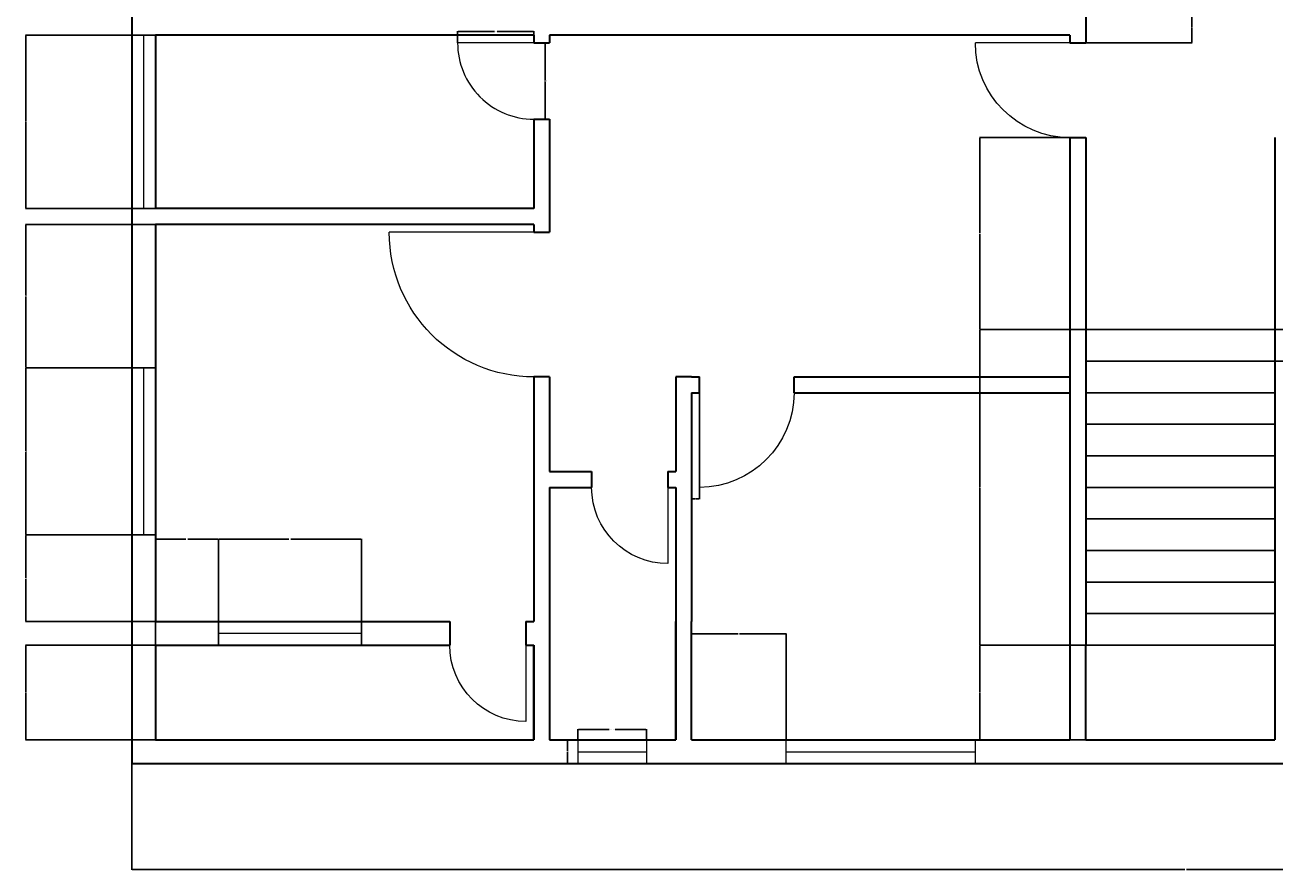
# Model space of a CAD drawing. Units: inches. Extents: x 2811 to 3694, y 2039 to 2670.
# Tile 1 of 3: x 2811 to 3286, y 2039 to 2361. Entities that reach past the tile are written whole.
import ezdxf

# ---------------------------------------------------------------- set-up
doc = ezdxf.new("R2010")
doc.units = ezdxf.units.IN
for name, color, linetype, lineweight in [('A-ANNO-DIMS', 2, 'Continuous', 18), ('A-DOOR', 3, 'Continuous', 18), ('A-FLOR-STRS', 2, 'Continuous', 25), ('A-GLAZ', 4, 'Continuous', 18), ('A-WALL', 7, 'Continuous', 35)]:
    doc.layers.add(name, color=color, linetype=linetype, lineweight=lineweight)
doc.styles.get("Standard").update_dxf_attribs({"font": 'arial.ttf'})
doc.dimstyles.get("Standard").update_dxf_attribs({"dimtxt": 0.18, "dimasz": 0.18, "dimexe": 0.18, "dimexo": 0.0625, "dimgap": 0.09, "dimtad": 0, "dimtih": 1, "dimtoh": 1, "dimdec": 4, "dimzin": 0, "dimdsep": 46, "dimtxsty": 'Standard', "dimcen": 0.09, "dimadec": 0, "dimazin": 0, "dimtfac": 1, "dimtdec": 4, "dimtofl": 0, "dimtmove": 0, "dimatfit": 3, "dimfxl": 1, "dimtolj": 1, "dimtzin": 0, "dimarcsym": 0})

# ---------------------------------------------------------------- blocks, each defined once
blk = doc.blocks.new('DOOR-SWING-29IN')
blk.add_line((29, 0), (29, 29))
blk.add_arc((29, 0), 29, 90, 180)
blk = doc.blocks.new('DOOR-SWING-36IN')
blk.add_line((36, 0), (0, 0))
blk.add_arc((36, 0), 36, 90, 180)
blk = doc.blocks.new('DOOR-SWING-55IN')
blk.add_line((0, 55), (55, 55))
blk.add_arc((0, 55), 55, 270, 0)
blk = doc.blocks.new('WIN-72IN')
for p, q in [((0, 0), (0, 9)), ((72, 0), (72, 9)), ((0, 4.5), (72, 4.5))]:
    blk.add_line(p, q)
blk = doc.blocks.new('WIN-66IN')
for p, q in [((0, 66), (9, 66)), ((4.5, 0), (4.5, 66)), ((0, 0), (9, 0))]:
    blk.add_line(p, q)
blk = doc.blocks.new('WIN-26_08IN')
for p, q in [((0, 0), (0, 9)), ((26.08, 0), (26.08, 9)), ((26.08, 4.5), (0, 4.5))]:
    blk.add_line(p, q)
blk = doc.blocks.new('*D8')
at = {"layer": 'A-ANNO-DIMS', "color": 0, "lineweight": -2, "transparency": 16777216}
for p, q in [((3004.34, 2353.98), (3008.81, 2353.98)), ((3008.63, 2353.8), (3008.63, 2339.66)), ((3008.63, 2325.16), (3008.63, 2339.3)), ((3004.34, 2324.98), (3008.81, 2324.98))]:
    blk.add_line(p, q, dxfattribs=at)
at = {"layer": 'A-ANNO-DIMS', "color": 0, "transparency": 16777216}
for points in [[(3008.6, 2353.8), (3008.66, 2353.8), (3008.63, 2353.98)], [(3008.6, 2325.16), (3008.66, 2325.16), (3008.63, 2324.98)]]:
    blk.add_solid(points, dxfattribs=at)
at = {"layer": 'Defpoints', "color": 0, "transparency": 16777216}
for p in [(3004.28, 2353.98), (3008.63, 2353.98), (3004.28, 2324.98)]:
    blk.add_point(p, dxfattribs=at)
at = {"layer": 'A-ANNO-DIMS', "color": 0, "transparency": 16777216, "insert": (3008.63, 2339.48), "char_height": 0.18, "attachment_point": 5}
blk.add_mtext('\\A1;DOOR 29 TYP.', dxfattribs=at)
blk = doc.blocks.new('*D9')
at = {"layer": 'A-ANNO-DIMS', "color": 0, "lineweight": -2, "transparency": 16777216}
for p, q in [((2975.28, 2354.04), (2975.28, 2358.51)), ((2975.46, 2358.33), (2989.25, 2358.33)), ((3004.1, 2358.33), (2990.31, 2358.33)), ((3004.28, 2354.04), (3004.28, 2358.51))]:
    blk.add_line(p, q, dxfattribs=at)
at = {"layer": 'A-ANNO-DIMS', "color": 0, "transparency": 16777216}
for points in [[(2975.46, 2358.36), (2975.46, 2358.3), (2975.28, 2358.33)], [(3004.1, 2358.36), (3004.1, 2358.3), (3004.28, 2358.33)]]:
    blk.add_solid(points, dxfattribs=at)
at = {"layer": 'Defpoints', "color": 0, "transparency": 16777216}
for p in [(2975.28, 2358.33), (2975.28, 2353.98), (3004.28, 2353.98)]:
    blk.add_point(p, dxfattribs=at)
at = {"layer": 'A-ANNO-DIMS', "color": 0, "transparency": 16777216, "insert": (2989.78, 2358.33), "char_height": 0.18, "attachment_point": 5}
blk.add_mtext('\\A1;29 TYP.', dxfattribs=at)
blk = doc.blocks.new('*D18')
at = {"layer": 'A-ANNO-DIMS', "color": 0, "lineweight": -2, "transparency": 16777216}
for p, q in [((3021.03, 2089.04), (3021.03, 2093.07)), ((3021.21, 2092.89), (3032.95, 2092.89)), ((3046.93, 2092.89), (3035.19, 2092.89)), ((3047.11, 2089.04), (3047.11, 2093.07))]:
    blk.add_line(p, q, dxfattribs=at)
at = {"layer": 'A-ANNO-DIMS', "color": 0, "transparency": 16777216}
for points in [[(3021.21, 2092.92), (3021.21, 2092.86), (3021.03, 2092.89)], [(3046.93, 2092.92), (3046.93, 2092.86), (3047.11, 2092.89)]]:
    blk.add_solid(points, dxfattribs=at)
at = {"layer": 'Defpoints', "color": 0, "transparency": 16777216}
for p in [(3021.03, 2092.89), (3021.03, 2088.98), (3047.11, 2088.98)]:
    blk.add_point(p, dxfattribs=at)
at = {"layer": 'A-ANNO-DIMS', "color": 0, "transparency": 16777216, "insert": (3034.07, 2092.89), "char_height": 0.18, "attachment_point": 5}
blk.add_mtext('\\A1;WINDOW 26 TYP.', dxfattribs=at)
blk = doc.blocks.new('*D19')
at = {"layer": 'A-ANNO-DIMS', "color": 0, "lineweight": -2, "transparency": 16777216}
for p, q in [((3020.97, 2088.98), (3016.94, 2088.98)), ((3017.12, 2088.8), (3017.12, 2084.66)), ((3017.12, 2080.16), (3017.12, 2084.3)), ((3020.97, 2079.98), (3016.94, 2079.98))]:
    blk.add_line(p, q, dxfattribs=at)
at = {"layer": 'A-ANNO-DIMS', "color": 0, "transparency": 16777216}
for points in [[(3017.09, 2088.8), (3017.15, 2088.8), (3017.12, 2088.98)], [(3017.09, 2080.16), (3017.15, 2080.16), (3017.12, 2079.98)]]:
    blk.add_solid(points, dxfattribs=at)
at = {"layer": 'Defpoints', "color": 0, "transparency": 16777216}
for p in [(3021.03, 2088.98), (3017.12, 2079.98), (3021.03, 2079.98)]:
    blk.add_point(p, dxfattribs=at)
at = {"layer": 'A-ANNO-DIMS', "color": 0, "transparency": 16777216, "insert": (3017.12, 2084.48), "char_height": 0.18, "attachment_point": 5}
blk.add_mtext('\\A1;9 TYP.', dxfattribs=at)
blk = doc.blocks.new('*D22')
at = {"layer": 'A-ANNO-DIMS', "color": 0, "lineweight": -2, "transparency": 16777216}
for p, q in [((2851.28, 2079.92), (2851.28, 2039.5)), ((3653.28, 2079.92), (3653.28, 2039.5)), ((2851.46, 2039.68), (3251.99, 2039.68)), ((3653.1, 2039.68), (3252.56, 2039.68))]:
    blk.add_line(p, q, dxfattribs=at)
at = {"layer": 'A-ANNO-DIMS', "color": 0, "transparency": 16777216}
for points in [[(2851.46, 2039.71), (2851.46, 2039.65), (2851.28, 2039.68)], [(3653.1, 2039.71), (3653.1, 2039.65), (3653.28, 2039.68)]]:
    blk.add_solid(points, dxfattribs=at)
at = {"layer": 'Defpoints', "color": 0, "transparency": 16777216}
for p in [(2851.28, 2079.98), (3653.28, 2079.98), (3653.28, 2039.68)]:
    blk.add_point(p, dxfattribs=at)
at = {"layer": 'A-ANNO-DIMS', "color": 0, "transparency": 16777216, "insert": (3252.28, 2039.68), "char_height": 0.18, "attachment_point": 5}
blk.add_mtext('\\A1;802', dxfattribs=at)
blk = doc.blocks.new('*D35')
at = {"layer": 'A-ANNO-DIMS', "color": 0, "lineweight": -2, "transparency": 16777216}
for p, q in [((2860.21, 2356.98), (2810.8, 2356.98)), ((2810.98, 2356.8), (2810.98, 2324.16)), ((2810.98, 2291.16), (2810.98, 2323.8)), ((2860.21, 2290.98), (2810.8, 2290.98))]:
    blk.add_line(p, q, dxfattribs=at)
at = {"layer": 'A-ANNO-DIMS', "color": 0, "transparency": 16777216}
for points in [[(2810.95, 2356.8), (2811.01, 2356.8), (2810.98, 2356.98)], [(2810.95, 2291.16), (2811.01, 2291.16), (2810.98, 2290.98)]]:
    blk.add_solid(points, dxfattribs=at)
at = {"layer": 'Defpoints', "color": 0, "transparency": 16777216}
for p in [(2860.28, 2356.98), (2810.98, 2290.98), (2860.28, 2290.98)]:
    blk.add_point(p, dxfattribs=at)
at = {"layer": 'A-ANNO-DIMS', "color": 0, "transparency": 16777216, "insert": (2810.98, 2323.98), "char_height": 0.18, "attachment_point": 5}
blk.add_mtext('\\A1;66', dxfattribs=at)
blk = doc.blocks.new('*D36')
at = {"layer": 'A-ANNO-DIMS', "color": 0, "lineweight": -2, "transparency": 16777216}
for p, q in [((2860.21, 2284.98), (2810.8, 2284.98)), ((2810.98, 2284.8), (2810.98, 2257.91)), ((2810.98, 2230.66), (2810.98, 2257.55)), ((2860.21, 2230.48), (2810.8, 2230.48))]:
    blk.add_line(p, q, dxfattribs=at)
at = {"layer": 'A-ANNO-DIMS', "color": 0, "transparency": 16777216}
for points in [[(2810.95, 2284.8), (2811.01, 2284.8), (2810.98, 2284.98)], [(2810.95, 2230.66), (2811.01, 2230.66), (2810.98, 2230.48)]]:
    blk.add_solid(points, dxfattribs=at)
at = {"layer": 'Defpoints', "color": 0, "transparency": 16777216}
for p in [(2860.28, 2284.98), (2810.98, 2230.48), (2860.28, 2230.48)]:
    blk.add_point(p, dxfattribs=at)
at = {"layer": 'A-ANNO-DIMS', "color": 0, "transparency": 16777216, "insert": (2810.98, 2257.73), "char_height": 0.18, "attachment_point": 5}
blk.add_mtext('\\A1;54.5', dxfattribs=at)
blk = doc.blocks.new('*D37')
at = {"layer": 'A-ANNO-DIMS', "color": 0, "lineweight": -2, "transparency": 16777216}
for p, q in [((2860.21, 2230.48), (2810.8, 2230.48)), ((2810.98, 2230.3), (2810.98, 2198.87)), ((2810.98, 2167.07), (2810.98, 2198.5)), ((2860.21, 2166.89), (2810.8, 2166.89))]:
    blk.add_line(p, q, dxfattribs=at)
at = {"layer": 'A-ANNO-DIMS', "color": 0, "transparency": 16777216}
for points in [[(2810.95, 2230.3), (2811.01, 2230.3), (2810.98, 2230.48)], [(2810.95, 2167.07), (2811.01, 2167.07), (2810.98, 2166.89)]]:
    blk.add_solid(points, dxfattribs=at)
at = {"layer": 'Defpoints', "color": 0, "transparency": 16777216}
for p in [(2860.28, 2230.48), (2810.98, 2166.89), (2860.28, 2166.89)]:
    blk.add_point(p, dxfattribs=at)
at = {"layer": 'A-ANNO-DIMS', "color": 0, "transparency": 16777216, "insert": (2810.98, 2198.68), "char_height": 0.18, "attachment_point": 5}
blk.add_mtext('\\A1;63.59', dxfattribs=at)
blk = doc.blocks.new('*D38')
at = {"layer": 'A-ANNO-DIMS', "color": 0, "lineweight": -2, "transparency": 16777216}
for p, q in [((2860.21, 2166.89), (2810.8, 2166.89)), ((2810.98, 2166.71), (2810.98, 2150.62)), ((2810.98, 2134.16), (2810.98, 2150.25)), ((2860.21, 2133.98), (2810.8, 2133.98))]:
    blk.add_line(p, q, dxfattribs=at)
at = {"layer": 'A-ANNO-DIMS', "color": 0, "transparency": 16777216}
for points in [[(2810.95, 2166.71), (2811.01, 2166.71), (2810.98, 2166.89)], [(2810.95, 2134.16), (2811.01, 2134.16), (2810.98, 2133.98)]]:
    blk.add_solid(points, dxfattribs=at)
at = {"layer": 'Defpoints', "color": 0, "transparency": 16777216}
for p in [(2860.28, 2166.89), (2810.98, 2133.98), (2860.28, 2133.98)]:
    blk.add_point(p, dxfattribs=at)
at = {"layer": 'A-ANNO-DIMS', "color": 0, "transparency": 16777216, "insert": (2810.98, 2150.43), "char_height": 0.18, "attachment_point": 5}
blk.add_mtext('\\A1;32.91', dxfattribs=at)
blk = doc.blocks.new('*D39')
at = {"layer": 'A-ANNO-DIMS', "color": 0, "lineweight": -2, "transparency": 16777216}
for p, q in [((2860.21, 2124.98), (2810.8, 2124.98)), ((2810.98, 2124.8), (2810.98, 2107.16)), ((2810.98, 2089.16), (2810.98, 2106.8)), ((2860.21, 2088.98), (2810.8, 2088.98))]:
    blk.add_line(p, q, dxfattribs=at)
at = {"layer": 'A-ANNO-DIMS', "color": 0, "transparency": 16777216}
for points in [[(2810.95, 2124.8), (2811.01, 2124.8), (2810.98, 2124.98)], [(2810.95, 2089.16), (2811.01, 2089.16), (2810.98, 2088.98)]]:
    blk.add_solid(points, dxfattribs=at)
at = {"layer": 'Defpoints', "color": 0, "transparency": 16777216}
for p in [(2860.28, 2124.98), (2810.98, 2088.98), (2860.28, 2088.98)]:
    blk.add_point(p, dxfattribs=at)
at = {"layer": 'A-ANNO-DIMS', "color": 0, "transparency": 16777216, "insert": (2810.98, 2106.98), "char_height": 0.18, "attachment_point": 5}
blk.add_mtext('\\A1;36', dxfattribs=at)
blk = doc.blocks.new('*D47')
at = {"layer": 'A-ANNO-DIMS', "color": 0, "lineweight": -2, "transparency": 16777216}
for p, q in [((2860.28, 2125.04), (2860.28, 2165.46)), ((2860.46, 2165.28), (2871.88, 2165.28)), ((2884.08, 2165.28), (2872.67, 2165.28)), ((2884.26, 2125.04), (2884.26, 2165.46))]:
    blk.add_line(p, q, dxfattribs=at)
at = {"layer": 'A-ANNO-DIMS', "color": 0, "transparency": 16777216}
for points in [[(2860.46, 2165.31), (2860.46, 2165.25), (2860.28, 2165.28)], [(2884.08, 2165.31), (2884.08, 2165.25), (2884.26, 2165.28)]]:
    blk.add_solid(points, dxfattribs=at)
at = {"layer": 'Defpoints', "color": 0, "transparency": 16777216}
for p in [(2884.26, 2165.28), (2860.28, 2124.98), (2884.26, 2124.98)]:
    blk.add_point(p, dxfattribs=at)
at = {"layer": 'A-ANNO-DIMS', "color": 0, "transparency": 16777216, "insert": (2872.27, 2165.28), "char_height": 0.18, "attachment_point": 5}
blk.add_mtext('\\A1;23.99', dxfattribs=at)
blk = doc.blocks.new('*D48')
at = {"layer": 'A-ANNO-DIMS', "color": 0, "lineweight": -2, "transparency": 16777216}
for p, q in [((2884.26, 2125.04), (2884.26, 2165.46)), ((2884.44, 2165.28), (2911.1, 2165.28)), ((2938.5, 2165.28), (2911.85, 2165.28)), ((2938.68, 2125.04), (2938.68, 2165.46))]:
    blk.add_line(p, q, dxfattribs=at)
at = {"layer": 'A-ANNO-DIMS', "color": 0, "transparency": 16777216}
for points in [[(2884.44, 2165.31), (2884.44, 2165.25), (2884.26, 2165.28)], [(2938.5, 2165.31), (2938.5, 2165.25), (2938.68, 2165.28)]]:
    blk.add_solid(points, dxfattribs=at)
at = {"layer": 'Defpoints', "color": 0, "transparency": 16777216}
for p in [(2938.68, 2165.28), (2884.26, 2124.98), (2938.68, 2124.98)]:
    blk.add_point(p, dxfattribs=at)
at = {"layer": 'A-ANNO-DIMS', "color": 0, "transparency": 16777216, "insert": (2911.47, 2165.28), "char_height": 0.18, "attachment_point": 5}
blk.add_mtext('\\A1;54.41', dxfattribs=at)
blk = doc.blocks.new('*D51')
at = {"layer": 'A-ANNO-DIMS', "color": 0, "lineweight": -2, "transparency": 16777216}
for p, q in [((3064.28, 2089.04), (3064.28, 2129.46)), ((3064.46, 2129.28), (3082.06, 2129.28)), ((3100.1, 2129.28), (3082.5, 2129.28)), ((3100.28, 2089.04), (3100.28, 2129.46))]:
    blk.add_line(p, q, dxfattribs=at)
at = {"layer": 'A-ANNO-DIMS', "color": 0, "transparency": 16777216}
for points in [[(3064.46, 2129.31), (3064.46, 2129.25), (3064.28, 2129.28)], [(3100.1, 2129.31), (3100.1, 2129.25), (3100.28, 2129.28)]]:
    blk.add_solid(points, dxfattribs=at)
at = {"layer": 'Defpoints', "color": 0, "transparency": 16777216}
for p in [(3100.28, 2129.28), (3064.28, 2088.98), (3100.28, 2088.98)]:
    blk.add_point(p, dxfattribs=at)
at = {"layer": 'A-ANNO-DIMS', "color": 0, "transparency": 16777216, "insert": (3082.28, 2129.28), "char_height": 0.18, "attachment_point": 5}
blk.add_mtext('\\A1;36', dxfattribs=at)
blk = doc.blocks.new('*D55')
at = {"layer": 'A-ANNO-DIMS', "color": 0, "lineweight": -2, "transparency": 16777216}
for p, q in [((3064.28, 2220.92), (3064.28, 2180.5)), ((3067.28, 2220.92), (3067.28, 2180.5)), ((3064.46, 2180.68), (3065.63, 2180.68)), ((3067.1, 2180.68), (3065.93, 2180.68))]:
    blk.add_line(p, q, dxfattribs=at)
at = {"layer": 'A-ANNO-DIMS', "color": 0, "transparency": 16777216}
for points in [[(3064.46, 2180.71), (3064.46, 2180.65), (3064.28, 2180.68)], [(3067.1, 2180.71), (3067.1, 2180.65), (3067.28, 2180.68)]]:
    blk.add_solid(points, dxfattribs=at)
at = {"layer": 'Defpoints', "color": 0, "transparency": 16777216}
for p in [(3064.28, 2220.98), (3067.28, 2220.98), (3064.28, 2180.68)]:
    blk.add_point(p, dxfattribs=at)
at = {"layer": 'A-ANNO-DIMS', "color": 0, "transparency": 16777216, "insert": (3065.78, 2180.68), "char_height": 0.18, "attachment_point": 5}
blk.add_mtext('\\A1;3', dxfattribs=at)
blk = doc.blocks.new('*D56')
at = {"layer": 'A-ANNO-DIMS', "color": 0, "lineweight": -2, "transparency": 16777216}
for p, q in [((3214.21, 2244.98), (3173.8, 2244.98)), ((3173.98, 2244.8), (3173.98, 2185.16)), ((3173.98, 2125.16), (3173.98, 2184.8)), ((3214.21, 2124.98), (3173.8, 2124.98))]:
    blk.add_line(p, q, dxfattribs=at)
at = {"layer": 'A-ANNO-DIMS', "color": 0, "transparency": 16777216}
for points in [[(3173.95, 2244.8), (3174.01, 2244.8), (3173.98, 2244.98)], [(3173.95, 2125.16), (3174.01, 2125.16), (3173.98, 2124.98)]]:
    blk.add_solid(points, dxfattribs=at)
at = {"layer": 'Defpoints', "color": 0, "transparency": 16777216}
for p in [(3173.98, 2244.98), (3214.28, 2244.98), (3214.28, 2124.98)]:
    blk.add_point(p, dxfattribs=at)
at = {"layer": 'A-ANNO-DIMS', "color": 0, "transparency": 16777216, "insert": (3173.98, 2184.98), "char_height": 0.18, "attachment_point": 5}
blk.add_mtext('\\A1;120', dxfattribs=at)
blk = doc.blocks.new('*D57')
at = {"layer": 'A-ANNO-DIMS', "color": 0, "lineweight": -2, "transparency": 16777216}
for p, q in [((3286.34, 2244.98), (3326.76, 2244.98)), ((3326.58, 2244.8), (3326.58, 2239.16)), ((3326.58, 2233.16), (3326.58, 2238.8)), ((3286.34, 2232.98), (3326.76, 2232.98))]:
    blk.add_line(p, q, dxfattribs=at)
at = {"layer": 'A-ANNO-DIMS', "color": 0, "transparency": 16777216}
for points in [[(3326.55, 2244.8), (3326.61, 2244.8), (3326.58, 2244.98)], [(3326.55, 2233.16), (3326.61, 2233.16), (3326.58, 2232.98)]]:
    blk.add_solid(points, dxfattribs=at)
at = {"layer": 'Defpoints', "color": 0, "transparency": 16777216}
for p in [(3286.28, 2244.98), (3286.28, 2232.98), (3326.58, 2232.98)]:
    blk.add_point(p, dxfattribs=at)
at = {"layer": 'A-ANNO-DIMS', "color": 0, "transparency": 16777216, "insert": (3326.58, 2238.98), "char_height": 0.18, "attachment_point": 5}
blk.add_mtext('\\A1;12', dxfattribs=at)
blk = doc.blocks.new('*D58')
at = {"layer": 'A-ANNO-DIMS', "color": 0, "lineweight": -2, "transparency": 16777216}
for p, q in [((3214.21, 2124.98), (3173.8, 2124.98)), ((3173.98, 2124.8), (3173.98, 2107.16)), ((3173.98, 2089.16), (3173.98, 2106.8)), ((3214.21, 2088.98), (3173.8, 2088.98))]:
    blk.add_line(p, q, dxfattribs=at)
at = {"layer": 'A-ANNO-DIMS', "color": 0, "transparency": 16777216}
for points in [[(3173.95, 2124.8), (3174.01, 2124.8), (3173.98, 2124.98)], [(3173.95, 2089.16), (3174.01, 2089.16), (3173.98, 2088.98)]]:
    blk.add_solid(points, dxfattribs=at)
at = {"layer": 'Defpoints', "color": 0, "transparency": 16777216}
for p in [(3173.98, 2124.98), (3214.28, 2124.98), (3214.28, 2088.98)]:
    blk.add_point(p, dxfattribs=at)
at = {"layer": 'A-ANNO-DIMS', "color": 0, "transparency": 16777216, "insert": (3173.98, 2106.98), "char_height": 0.18, "attachment_point": 5}
blk.add_mtext('\\A1;36', dxfattribs=at)
blk = doc.blocks.new('*D59')
at = {"layer": 'A-ANNO-DIMS', "color": 0, "lineweight": -2, "transparency": 16777216}
for p, q in [((3214.21, 2317.98), (3173.8, 2317.98)), ((3173.98, 2317.8), (3173.98, 2281.66)), ((3173.98, 2245.16), (3173.98, 2281.3)), ((3214.21, 2244.98), (3173.8, 2244.98))]:
    blk.add_line(p, q, dxfattribs=at)
at = {"layer": 'A-ANNO-DIMS', "color": 0, "transparency": 16777216}
for points in [[(3173.95, 2317.8), (3174.01, 2317.8), (3173.98, 2317.98)], [(3173.95, 2245.16), (3174.01, 2245.16), (3173.98, 2244.98)]]:
    blk.add_solid(points, dxfattribs=at)
at = {"layer": 'Defpoints', "color": 0, "transparency": 16777216}
for p in [(3173.98, 2317.98), (3214.28, 2317.98), (3214.28, 2244.98)]:
    blk.add_point(p, dxfattribs=at)
at = {"layer": 'A-ANNO-DIMS', "color": 0, "transparency": 16777216, "insert": (3173.98, 2281.48), "char_height": 0.18, "attachment_point": 5}
blk.add_mtext('\\A1;73', dxfattribs=at)
blk = doc.blocks.new('*D62')
at = {"layer": 'A-ANNO-DIMS', "color": 0, "lineweight": -2, "transparency": 16777216}
for p, q in [((3214.34, 2365.98), (3254.76, 2365.98)), ((3254.58, 2365.8), (3254.58, 2360.16)), ((3254.58, 2354.16), (3254.58, 2359.8)), ((3214.34, 2353.98), (3254.76, 2353.98))]:
    blk.add_line(p, q, dxfattribs=at)
at = {"layer": 'A-ANNO-DIMS', "color": 0, "transparency": 16777216}
for points in [[(3254.55, 2365.8), (3254.61, 2365.8), (3254.58, 2365.98)], [(3254.55, 2354.16), (3254.61, 2354.16), (3254.58, 2353.98)]]:
    blk.add_solid(points, dxfattribs=at)
at = {"layer": 'Defpoints', "color": 0, "transparency": 16777216}
for p in [(3214.28, 2365.98), (3214.28, 2353.98), (3254.58, 2353.98)]:
    blk.add_point(p, dxfattribs=at)
at = {"layer": 'A-ANNO-DIMS', "color": 0, "transparency": 16777216, "insert": (3254.58, 2359.98), "char_height": 0.18, "attachment_point": 5}
blk.add_mtext('\\A1;12', dxfattribs=at)

msp = doc.modelspace()

# ---------------------------------------------------------------- linework, layer by layer
at = {"layer": 'A-FLOR-STRS'}
for p, q in [((3214.2765, 2244.9792), (3286.2765, 2244.9792)), ((3214.2765, 2232.9792), (3286.2765, 2232.9792)), ((3214.2765, 2220.9792), (3286.2765, 2220.9792)), ((3214.2765, 2208.9792), (3286.2765, 2208.9792)), ((3214.2765, 2196.9792), (3286.2765, 2196.9792)), ((3214.2765, 2184.9792), (3286.2765, 2184.9792)), ((3214.2765, 2172.9792), (3286.2765, 2172.9792)), ((3214.2765, 2160.9792), (3286.2765, 2160.9792)), ((3214.2765, 2148.9792), (3286.2765, 2148.9792)), ((3214.2765, 2136.9792), (3286.2765, 2136.9792)), ((3214.2765, 2124.9792), (3286.2765, 2124.9792)), ((3214.2765, 2124.9792), (3286.2765, 2124.9792))]:
    msp.add_line(p, q, dxfattribs=at)
at = {"layer": 'A-GLAZ'}
for p, q in [((2851.2765, 2290.9792), (2851.2765, 2356.9792)), ((2851.2765, 2166.8907), (2851.2765, 2230.4792)), ((2851.2765, 2230.4792), (2860.2765, 2230.4792)), ((2860.2765, 2230.4792), (2855.7765, 2230.4792)), ((2855.7765, 2230.4792), (2855.7765, 2166.8907)), ((2860.2765, 2166.8907), (2851.2765, 2166.8907)), ((2884.2647, 2133.9792), (2884.2647, 2124.9792)), ((2938.6787, 2124.9792), (2938.6787, 2133.9792)), ((2938.6787, 2133.9792), (2938.6787, 2129.4792)), ((2938.6787, 2129.4792), (2884.2647, 2129.4792)), ((2884.2647, 2124.9792), (2938.6787, 2124.9792)), ((3021.0309, 2079.9792), (3047.1112, 2079.9792)), ((3100.2765, 2079.9792), (3172.2765, 2079.9792))]:
    msp.add_line(p, q, dxfattribs=at)
at = {"layer": 'A-WALL'}
for p, q in [((2851.2765, 2629.9792), (2851.2765, 2124.9792)), ((3214.2765, 2365.9792), (3214.2765, 2353.9792)), ((2860.2765, 2356.9792), (2860.2765, 2290.9792)), ((3004.2765, 2356.9792), (2860.2765, 2356.9792)), ((3004.2765, 2356.9792), (3004.2765, 2353.9792)), ((3208.2765, 2356.9792), (3010.2765, 2356.9792)), ((3010.2765, 2356.9792), (3010.2765, 2353.9792)), ((3208.2765, 2356.9792), (3208.2765, 2353.9792)), ((3004.2765, 2353.9792), (3010.2765, 2353.9792)), ((3208.2765, 2353.9792), (3214.2765, 2353.9792)), ((3004.2765, 2324.9792), (3010.2765, 2324.9792)), ((3004.2765, 2324.9792), (3004.2765, 2290.9792)), ((3010.2765, 2324.9792), (3010.2765, 2281.9792)), ((3208.2765, 2317.9792), (3214.2765, 2317.9792)), ((3208.2765, 2317.9792), (3208.2765, 2271.9792)), ((3214.2765, 2317.9792), (3214.2765, 2133.9792)), ((3286.2765, 2317.9792), (3286.2765, 2133.9792)), ((3004.2765, 2290.9792), (2860.2765, 2290.9792)), ((3004.2765, 2284.9792), (2860.2765, 2284.9792)), ((2860.2765, 2284.9792), (2860.2765, 2175.9792)), ((3004.2765, 2284.9792), (3004.2765, 2281.9792)), ((3004.2765, 2281.9792), (3010.2765, 2281.9792)), ((3208.2765, 2271.9792), (3208.2765, 2265.9792)), ((3208.2765, 2265.9792), (3208.2765, 2133.9792)), ((3004.2765, 2226.9792), (3004.2765, 2175.9792)), ((3010.2765, 2226.9792), (3004.2765, 2226.9792)), ((3010.2765, 2226.9792), (3010.2765, 2190.9792)), ((3058.2765, 2226.9792), (3058.2765, 2190.9792)), ((3064.2765, 2226.9792), (3058.2765, 2226.9792)), ((3064.2765, 2226.9792), (3067.2765, 2226.9792)), ((3067.2765, 2220.9792), (3067.2765, 2226.9792)), ((3103.2765, 2220.9792), (3103.2765, 2226.9792)), ((3103.2765, 2226.9792), (3208.2765, 2226.9792)), ((3064.2765, 2220.9792), (3064.2765, 2133.9792)), ((3064.2765, 2220.9792), (3067.2765, 2220.9792)), ((3103.2765, 2220.9792), (3208.2765, 2220.9792)), ((3010.2765, 2190.9792), (3026.2765, 2190.9792)), ((3026.2765, 2190.9792), (3026.2765, 2184.9792)), ((3055.2765, 2190.9792), (3055.2765, 2184.9792)), ((3055.2765, 2190.9792), (3058.2765, 2190.9792)), ((3010.2765, 2184.9792), (3026.2765, 2184.9792)), ((3010.2765, 2184.9792), (3010.2765, 2133.9792)), ((3055.2765, 2184.9792), (3058.2765, 2184.9792)), ((3058.2765, 2184.9792), (3058.2765, 2133.9792)), ((2860.2765, 2175.9792), (2860.2765, 2166.8907)), ((3004.2765, 2175.9792), (3004.2765, 2167.4365)), ((2860.2765, 2169.9792), (2860.2765, 2133.9792)), ((3004.2765, 2169.9792), (3004.2765, 2133.9792)), ((2860.2765, 2133.9792), (2972.2765, 2133.9792)), ((2972.2765, 2133.9792), (2972.2765, 2124.9792)), ((3001.2765, 2133.9792), (3001.2765, 2124.9792)), ((3001.2765, 2133.9792), (3004.2765, 2133.9792)), ((3010.2765, 2133.9792), (3010.2765, 2088.9792)), ((3058.2765, 2088.9792), (3058.2765, 2133.9792)), ((3058.2765, 2133.9792), (3058.2765, 2088.9792)), ((3064.2765, 2088.9792), (3064.2765, 2133.9792)), ((3208.2765, 2133.9792), (3208.2765, 2088.9792)), ((3214.2765, 2133.9792), (3214.2765, 2124.9792)), ((3286.2765, 2133.9792), (3286.2765, 2124.9792)), ((2851.2765, 2124.9792), (2851.2765, 2079.9792)), ((2860.2765, 2124.9792), (2972.2765, 2124.9792)), ((2860.2765, 2124.9792), (2860.2765, 2088.9792)), ((3001.2765, 2124.9792), (3004.2765, 2124.9792)), ((3004.2765, 2088.9792), (3004.2765, 2124.9792)), ((3004.2765, 2124.9792), (3004.2765, 2088.9792)), ((3214.2765, 2088.9792), (3214.2765, 2124.9792)), ((3286.2765, 2124.9792), (3286.2765, 2088.9792)), ((2860.2765, 2088.9792), (3004.2765, 2088.9792)), ((3010.2765, 2088.9792), (3058.2765, 2088.9792)), ((3010.2765, 2088.9792), (3058.2765, 2088.9792)), ((3064.2765, 2088.9792), (3208.2765, 2088.9792)), ((3214.2765, 2088.9792), (3286.2765, 2088.9792)), ((2851.2765, 2079.9792), (3653.2765, 2079.9792))]:
    msp.add_line(p, q, dxfattribs=at)

# ---------------------------------------------------------------- block references
at = {"layer": 'A-DOOR', "rotation": 90.0000000000009}
msp.add_blockref('DOOR-SWING-29IN', (3004.2768, 2324.9797), dxfattribs=at)
at = {"layer": 'A-DOOR', "extrusion": (0, 0, -1), "zscale": -1}
for name, p, rotation in [('DOOR-SWING-36IN', (-3172.277, 2353.9795), 180), ('DOOR-SWING-36IN', (-3067.2763, 2184.9797), 89.99999999999964), ('DOOR-SWING-29IN', (-3026.277, 2184.9795), 180), ('DOOR-SWING-29IN', (-2972.277, 2124.9795), 180)]:
    msp.add_blockref(name, p, dxfattribs=dict(at, rotation=rotation))
msp.add_blockref('DOOR-SWING-55IN', (-3004.2761, 2226.979), dxfattribs=at)
at = {"layer": 'A-GLAZ', "rotation": 180}
for name, p in [('WIN-66IN', (2860.2761, 2356.9795)), ('WIN-26_08IN', (3047.1111, 2088.9795))]:
    msp.add_blockref(name, p, dxfattribs=at)
at = {"layer": 'A-GLAZ'}
msp.add_blockref('WIN-72IN', (3100.277, 2079.979), dxfattribs=at)

# ---------------------------------------------------------------- dimensions: what is measured, and where the dimension line sits
at = {"layer": 'A-ANNO-DIMS'}
for base, p1, p2, angle, override, picture, middle in [((3254.5765, 2353.9792), (3214.2765, 2365.9792), (3214.2765, 2353.9792), 270, {"dimdec": 0, "dimlfac": 1, "dimrnd": 0, "dimzin": 0, "dimdsep": 46, "dimlunit": 2}, '*D62', (3254.5765, 2359.9792)), ((2810.9765, 2290.9792), (2860.2765, 2356.9792), (2860.2765, 2290.9792), 90, {"dimdec": 0, "dimlfac": 1, "dimrnd": 0, "dimzin": 0, "dimdsep": 46, "dimlunit": 2}, '*D35', (2810.9765, 2323.9792)), ((3173.9765, 2317.9792), (3214.2765, 2244.9792), (3214.2765, 2317.9792), 90, {"dimdec": 0, "dimlfac": 1, "dimrnd": 0, "dimzin": 0, "dimdsep": 46, "dimlunit": 2}, '*D59', (3173.9765, 2281.4792)), ((2810.9765, 2230.4792), (2860.2765, 2284.9792), (2860.2765, 2230.4792), 90, {"dimdec": 1, "dimlfac": 1, "dimrnd": 0, "dimzin": 0, "dimdsep": 46, "dimlunit": 2}, '*D36', (2810.9765, 2257.7292)), ((3173.9765, 2244.9792), (3214.2765, 2124.9792), (3214.2765, 2244.9792), 90, {"dimdec": 0, "dimlfac": 1, "dimrnd": 0, "dimzin": 0, "dimdsep": 46, "dimlunit": 2}, '*D56', (3173.9765, 2184.9792)), ((3326.5765, 2232.9792), (3286.2765, 2244.9792), (3286.2765, 2232.9792), 270, {"dimdec": 0, "dimlfac": 1, "dimrnd": 0, "dimzin": 0, "dimdsep": 46, "dimlunit": 2}, '*D57', (3326.5765, 2238.9792)), ((2810.9765, 2166.8907), (2860.2765, 2230.4792), (2860.2765, 2166.8907), 90, {"dimdec": 2, "dimlfac": 1, "dimrnd": 0, "dimzin": 0, "dimdsep": 46, "dimlunit": 2}, '*D37', (2810.9765, 2198.685)), ((3064.2765, 2180.6792), (3067.2765, 2220.9792), (3064.2765, 2220.9792), 180, {"dimdec": 0, "dimlfac": 1, "dimrnd": 0, "dimzin": 0, "dimdsep": 46, "dimlunit": 2}, '*D55', (3065.7765, 2180.6792)), ((2810.9765, 2133.9792), (2860.2765, 2166.8907), (2860.2765, 2133.9792), 90, {"dimdec": 2, "dimlfac": 1, "dimrnd": 0, "dimzin": 0, "dimdsep": 46, "dimlunit": 2}, '*D38', (2810.9765, 2150.435)), ((2810.9765, 2088.9792), (2860.2765, 2124.9792), (2860.2765, 2088.9792), 90, {"dimdec": 0, "dimlfac": 1, "dimrnd": 0, "dimzin": 0, "dimdsep": 46, "dimlunit": 2}, '*D39', (2810.9765, 2106.9792)), ((3173.9765, 2124.9792), (3214.2765, 2088.9792), (3214.2765, 2124.9792), 90, {"dimdec": 0, "dimlfac": 1, "dimrnd": 0, "dimzin": 0, "dimdsep": 46, "dimlunit": 2}, '*D58', (3173.9765, 2106.9792))]:
    dim = msp.add_linear_dim(base=base, p1=p1, p2=p2, angle=angle, dimstyle='Standard', override=override, dxfattribs=at)
    dim.commit()
    dim.dimension.update_dxf_attribs({"geometry": picture, "text_midpoint": middle})
for base, p1, p2, angle, text, picture, middle in [((2975.2765, 2358.3292), (3004.2765, 2353.9792), (2975.2765, 2353.9792), 180, '<> TYP.', '*D9', (2989.7765, 2358.3292)), ((3008.6265, 2353.9792), (3004.2765, 2324.9792), (3004.2765, 2353.9792), 90, 'DOOR <> TYP.', '*D8', (3008.6265, 2339.4792)), ((3021.0309, 2092.8913), (3047.1112, 2088.9792), (3021.0309, 2088.9792), 180, 'WINDOW <> TYP.', '*D18', (3034.0711, 2092.8913)), ((3017.1189, 2079.9792), (3021.0309, 2088.9792), (3021.0309, 2079.9792), 270, '<> TYP.', '*D19', (3017.1189, 2084.4792))]:
    dim = msp.add_linear_dim(base=base, p1=p1, p2=p2, angle=angle, text=text, dimstyle='Standard', override={"dimdec": 0, "dimlfac": 1, "dimrnd": 0, "dimzin": 0, "dimdsep": 46, "dimlunit": 2}, dxfattribs=at)
    dim.commit()
    dim.dimension.update_dxf_attribs({"geometry": picture, "text_midpoint": middle})
for base, p1, p2, override, picture, middle in [((2884.2647, 2165.2792), (2860.2765, 2124.9792), (2884.2647, 2124.9792), {"dimdec": 2, "dimlfac": 1, "dimrnd": 0, "dimzin": 0, "dimdsep": 46, "dimlunit": 2}, '*D47', (2872.2706, 2165.2792)), ((2938.6787, 2165.2792), (2884.2647, 2124.9792), (2938.6787, 2124.9792), {"dimdec": 2, "dimlfac": 1, "dimrnd": 0, "dimzin": 0, "dimdsep": 46, "dimlunit": 2}, '*D48', (2911.4717, 2165.2792)), ((3100.2765, 2129.2792), (3064.2765, 2088.9792), (3100.2765, 2088.9792), {"dimdec": 0, "dimlfac": 1, "dimrnd": 0, "dimzin": 0, "dimdsep": 46, "dimlunit": 2}, '*D51', (3082.2765, 2129.2792)), ((3653.2765, 2039.6792), (2851.2765, 2079.9792), (3653.2765, 2079.9792), {"dimdec": 0, "dimlfac": 1, "dimrnd": 0, "dimzin": 0, "dimdsep": 46, "dimlunit": 2}, '*D22', (3252.2765, 2039.6792))]:
    dim = msp.add_linear_dim(base=base, p1=p1, p2=p2, dimstyle='Standard', override=override, dxfattribs=at)
    dim.commit()
    dim.dimension.update_dxf_attribs({"geometry": picture, "text_midpoint": middle})

doc.saveas('drawing.dxf')
